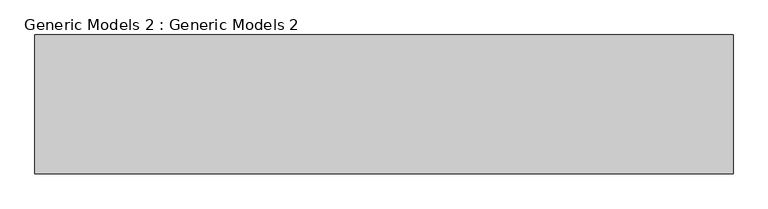
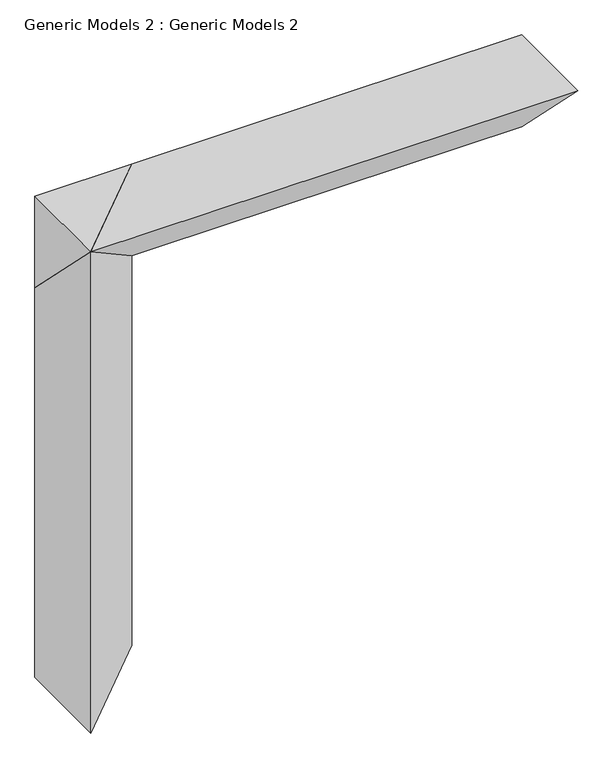
"""IFC4 building model written with IfcOpenShell, lengths in millimetres: proxy geometry, Generic Models 2 : Generic Models 2."""

from ifc_helpers import new_model, si_unit, frame, origin, place, context, project, spatial, polyline, outline, extrude, source, transform, mapped, element, save


def generic_models_2_generic_models_2_bb9d770e(model_context):
    return source(origin(), model_context, "Body", "SweptSolid", [
        extrude(outline(polyline([(-7961.058484, 6096.0), (-8570.658484, 6705.6), (-7961.058484, 6705.6), (-7961.058484, 6096.0)])), frame((-4855.6350579, 0.0, 0.0), z_axis=(1.0, 0.0, 0.0), x_axis=(0.0, 1.0, 0.0)), (0.0, 0.0, 1.0), 3062.8408029),
        extrude(outline(polyline([(-4246.0350579, -7961.058484), (-4855.6350579, -8570.658484), (-4855.6350579, -7961.058484), (-4246.0350579, -7961.058484)])), frame((0.0, 0.0, 3505.2), z_axis=(0.0, 0.0, 1.0), x_axis=(1.0, 0.0, 0.0)), (0.0, 0.0, 1.0), 3200.4),
    ])


if __name__ == "__main__":
    model = new_model("IFC4")
    model_context = context("Model", 3, world=origin())
    ifc_project = project(units=[si_unit("LENGTHUNIT", "METRE", prefix="MILLI")], contexts=[model_context])
    site = spatial("IfcSite", under=ifc_project)
    building = spatial("IfcBuilding", under=site)
    placement = place(None, origin())
    generic_models_2_generic_models_2_shape = generic_models_2_generic_models_2_bb9d770e(model_context)
    element("IfcBuildingElementProxy", 1, Name="Generic Models 2 : Generic Models 2", ObjectType="Generic Models 2 : Generic Models 2", at=placement, inside=building, context=model_context, shape_type="MappedRepresentation", body=[
        mapped(generic_models_2_generic_models_2_shape, transform((0.0, 0.0, 0.0), x_axis=(1.0, 0.0, 0.0), y_axis=(0.0, 1.0, 0.0), z_axis=(0.0, 0.0, 1.0))),
    ])
    save(model, "model.ifc")
